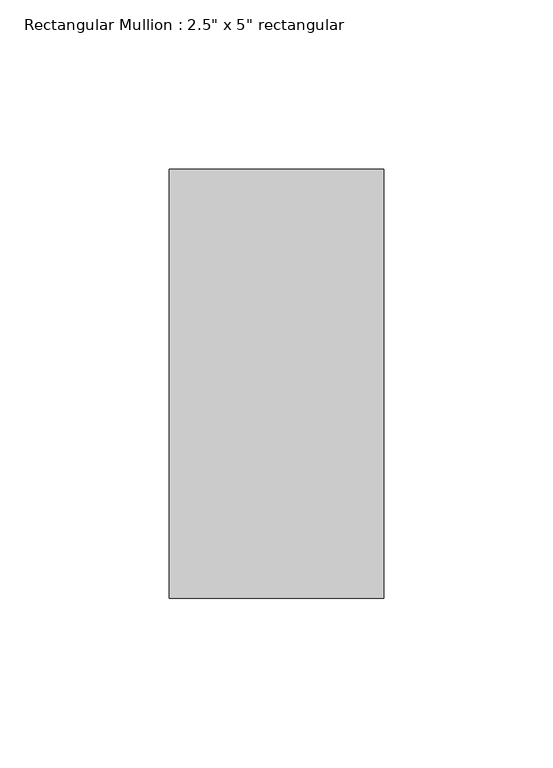
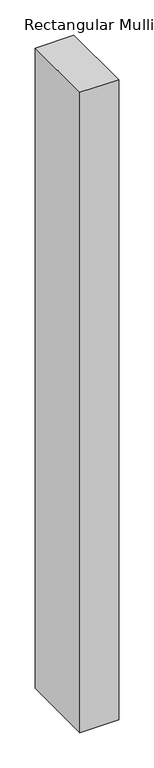
"""IFC4 building model written with IfcOpenShell, lengths in millimetres: member geometry."""

from ifc_helpers import new_model, si_unit, frame, origin, place, context, project, spatial, polyline, outline, extrude, source, transform, mapped, element, save


def member_48e25eb9(model_context):
    return source(origin(), model_context, "Body", "SweptSolid", [
        extrude(outline(polyline([(0.0, 63.5), (0.0, -63.5), (-63.5, -63.5), (-63.5, 63.5), (0.0, 63.5)])), frame((0.0, 0.0, -1110.6251745), z_axis=(0.0, 0.0, 1.0), x_axis=(1.0, 0.0, 0.0)), (0.0, 0.0, 1.0), 1110.6251745),
    ])


if __name__ == "__main__":
    model = new_model("IFC4")
    model_context = context("Model", 3, world=origin())
    ifc_project = project(units=[si_unit("LENGTHUNIT", "METRE", prefix="MILLI")], contexts=[model_context])
    site = spatial("IfcSite", under=ifc_project)
    building = spatial("IfcBuilding", under=site)
    placement = place(None, origin())
    member_shape = member_48e25eb9(model_context)
    element("IfcMember", 1, ObjectType="Rectangular Mullion : 2.5\" x 5\" rectangular", at=placement, inside=building, context=model_context, shape_type="MappedRepresentation", body=[
        mapped(member_shape, transform((0.0, 0.0, 0.0), x_axis=(1.0, 0.0, 0.0), y_axis=(0.0, 1.0, 0.0), z_axis=(0.0, 0.0, 1.0))),
    ])
    save(model, "model.ifc")

# Revit data of these elements
# Type "Rectangular Mullion : 2.5\" x 5\" rectangular"
#   built-in parameter 1007304 = 0.416667 (stored number, unit not read)
#   built-in parameter 1007301 = 0.104167 (stored number, unit not read)
#   built-in parameter 1007300 = 0.104167 (stored number, unit not read)
# Element 1 (IfcMember, "Rectangular Mullion : 2.5\" x 5\" rectangular")
#   Materials on its faces: "Aluminum"
# Materials
#   "Aluminum": class "Metal", colour RGB 247 247 247, transparency 0, Description = "Aluminum 6061", Cost = 0
